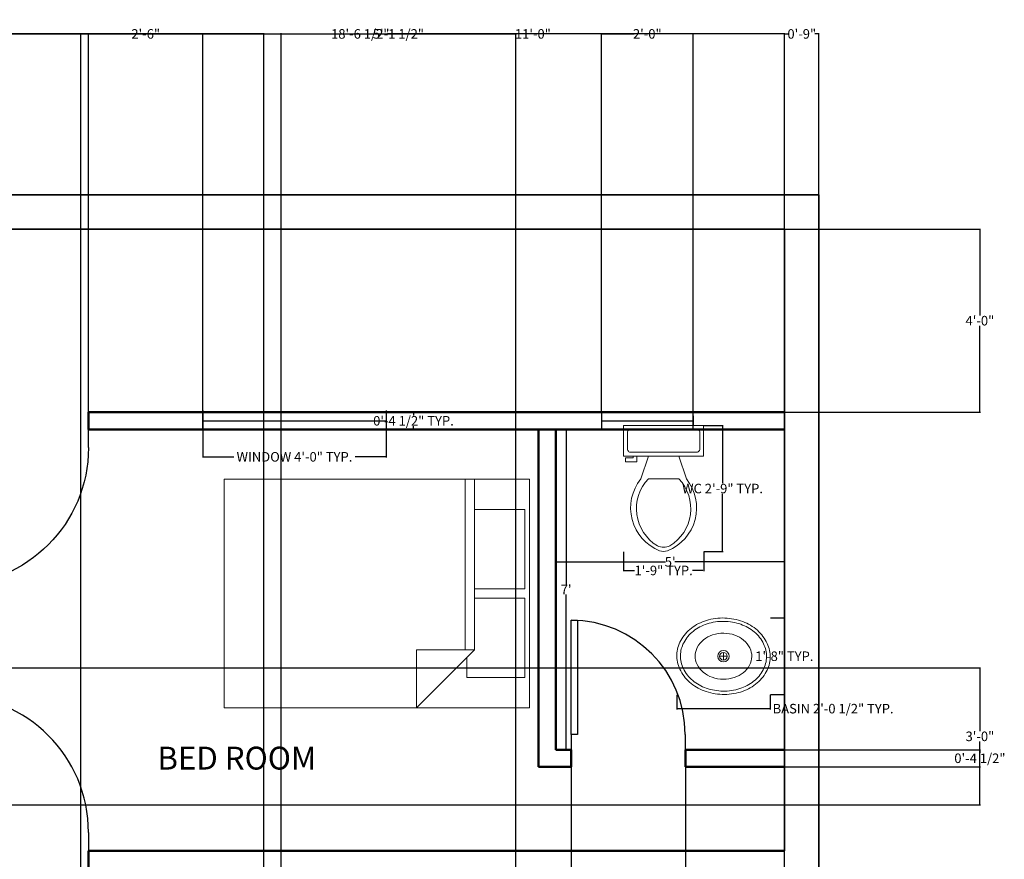
# Model space of a CAD drawing. Units: inches. Extents: x 594 to 1173, y 353 to 1285.
# Tile 6 of 6: x 914 to 1172, y 1065 to 1285. Entities that reach past the tile are written whole.
import ezdxf

# ---------------------------------------------------------------- set-up
doc = ezdxf.new("R2010")
doc.units = ezdxf.units.IN
doc.header["$MEASUREMENT"] = 0
for name, color, linetype, lineweight in [('A-ANNO-DIMS', 2, 'Continuous', 18), ('A-AREA-IDEN', 7, 'Continuous', 25), ('A-DOOR', 4, 'Continuous', 25), ('A-FLOR-FIXT', 9, 'Continuous', 18), ('A-FURN', 8, 'Continuous', 18), ('A-GLAZ', 4, 'Continuous', 25), ('A-WALL', 7, 'Continuous', 50), ('C-PROP', 7, 'Continuous', 35)]:
    doc.layers.add(name, color=color, linetype=linetype, lineweight=lineweight)
doc.styles.get("Standard").update_dxf_attribs({"font": 'arial.ttf'})
doc.dimstyles.get("Standard").update_dxf_attribs({"dimtxt": 2.5, "dimasz": 0.18, "dimexe": 0.18, "dimexo": 0.0625, "dimgap": 0.09, "dimtad": 0, "dimtih": 1, "dimtoh": 1, "dimzin": 0, "dimdsep": 46, "dimlunit": 3, "dimtxsty": 'Standard', "dimcen": 0.09, "dimadec": 0, "dimazin": 0, "dimtfac": 1, "dimtofl": 0, "dimtmove": 0, "dimatfit": 3, "dimfxl": 1, "dimtolj": 1, "dimtzin": 0, "dimarcsym": 0})

# ---------------------------------------------------------------- blocks, each defined once
blk = doc.blocks.new('*U4')
for p, q in [((0, 100), (0, 0)), ((900, 100), (900, 0)), ((0, 50), (900, 50))]:
    blk.add_line(p, q)
blk = doc.blocks.new('*U2')
for p, q in [((0, 0), (0, -100)), ((750, 0), (750, -100))]:
    blk.add_line(p, q)
blk.add_lwpolyline([(0, 0), (0, 750), (43.75, 750), (43.75, 0)], close=True)
blk.add_arc((0, 0), 750, 0, 90)
blk = doc.blocks.new('Bed - Queen')
for p, q in [((0, -80.00003), (0, 0)), ((0, 0), (59.99999, 0)), ((59.99999, 0), (59.99999, -80.00003)), ((7.99999, -1.2), (28.79998, -1.2)), ((7.99999, -14.4), (7.99999, -1.2)), ((28.79998, -1.2), (28.79998, -14.4)), ((31.19999, -1.2), (51.99999, -1.2)), ((31.19999, -14.4), (31.19999, -1.2)), ((51.99999, -1.2), (51.99999, -16.4)), ((0, -14.4), (44.8, -14.4)), ((59.99999, -29.6), (44.8, -14.4)), ((44.8, -14.4), (44.8, -29.6)), ((44.8, -16.8), (0, -16.8)), ((51.99999, -16.4), (46.79936, -16.4)), ((44.8, -29.6), (59.99999, -29.6)), ((59.99999, -80.00003), (0, -80.00003))]:
    blk.add_line(p, q)
blk = doc.blocks.new('Toilet - top')
for p, q in [((9.5, -6), (9.5, -2)), ((-10, -8.5), (-8, -8.5)), ((-10, -9.5), (-10, -8.5)), ((-7, -9.5), (-10, -9.5)), ((-8, -8.5), (-8, -8)), ((-7, -8), (-7, -9.5)), ((-4, -8), (-6, -14)), ((4, -8), (6, -14)), ((4, -14), (-4, -14))]:
    blk.add_line(p, q)
blk.add_lwpolyline([(10.5, -8), (10.5, 0), (-10.5, 0), (-10.5, -8)], close=True)
for points in [[(-9.5, -2), (-9.5, -6)], [(8.5, -1), (-8.5, -1)], [(-8.5, -7), (8.5, -7)]]:
    blk.add_lwpolyline(points)
for centre, radius, start, end in [((-8.62, -1.88), 0.884, 81.8699, 188.1301), ((8.62, -1.88), 0.884, 351.8699, 98.1301), ((-8.62, -6.12), 0.884, 171.8699, 278.1301), ((8.62, -6.12), 0.884, 261.8699, 8.1301), ((3.52, -21.58), 12.17, 141.4691, 247.9714), ((4.2, -21.82), 11.33, 136.3677, 238.9468), ((-3.52, -21.58), 12.17, 292.0284, 38.5307), ((-4.2, -21.82), 11.33, 301.053, 43.6321), ((0, -27.88), 4, 245.7318, 294.2682), ((0, -29), 4, 254.8605, 285.1395)]:
    blk.add_arc(centre, radius, start, end)
blk = doc.blocks.new('Sink - Oval top')
for p, q in [((-1, 0), (1, 0)), ((0, 1), (0, -1))]:
    blk.add_line(p, q)
for points in [[(-12.23, 0.39, 0.117634), (-11.46, -3.36, 0.104469), (-8.88, -6.8, 0.090016), (-5.08, -9.07, 0.08192), (-0.32, -10.02, 0.08192), (4.49, -9.38, 0.090016), (8.42, -7.36, 0.104469), (11.22, -4.09, 0.117634), (12.23, -0.39, 0.117634), (11.46, 3.36, 0.104469), (8.88, 6.8, 0.090016), (5.08, 9.07, 0.08192), (0.32, 10.02, 0.08192), (-4.49, 9.38, 0.090016), (-8.42, 7.36, 0.104469), (-11.22, 4.09, 0.117634)], [(-11.29, 0.16, 0.118622), (-10.52, -3.25, 0.104678), (-8.07, -6.36, 0.089562), (-4.54, -8.37, 0.081185), (-0.13, -9.15, 0.081185), (4.3, -8.49, 0.089562), (7.89, -6.58, 0.104678), (10.42, -3.55, 0.118622), (11.29, -0.16, 0.118622), (10.52, 3.25, 0.104678), (8.07, 6.36, 0.089562), (4.54, 8.37, 0.081185), (0.13, 9.15, 0.081185), (-4.3, 8.49, 0.089562), (-7.89, 6.58, 0.104678), (-10.42, 3.55, 0.118622)], [(-7.42, 0.08, 0.118283), (-6.91, -2.17, 0.104607), (-5.29, -4.21, 0.089718), (-2.97, -5.53, 0.081436), (-0.07, -6.04, 0.081436), (2.84, -5.59, 0.089718), (5.2, -4.33, 0.104607), (6.86, -2.32, 0.118283), (7.42, -0.08, 0.118283), (6.91, 2.17, 0.104607), (5.29, 4.21, 0.089718), (2.97, 5.53, 0.081436), (0.07, 6.04, 0.081436), (-2.84, 5.59, 0.089718), (-5.2, 4.33, 0.104607), (-6.86, 2.32, 0.118283)]]:
    blk.add_lwpolyline(points, format="xyb", close=True)
for radius in [1.5, 1]:
    blk.add_circle((0, 0), radius)
blk = doc.blocks.new('*D15')
at = {"layer": 'A-ANNO-DIMS', "color": 0, "lineweight": -2, "transparency": 16777216}
for p, q in [((1054.34, 1177.22), (1054.34, 1142.36)), ((1114.34, 1177.22), (1114.34, 1142.36)), ((1054.52, 1142.54), (1083.1, 1142.54)), ((1114.16, 1142.54), (1085.58, 1142.54))]:
    blk.add_line(p, q, dxfattribs=at)
at = {"layer": 'A-ANNO-DIMS', "color": 0, "transparency": 16777216}
for points in [[(1054.52, 1142.57), (1054.52, 1142.51), (1054.34, 1142.54)], [(1114.16, 1142.57), (1114.16, 1142.51), (1114.34, 1142.54)]]:
    blk.add_solid(points, dxfattribs=at)
at = {"layer": 'Defpoints', "color": 0, "transparency": 16777216}
for p in [(1054.34, 1177.28), (1114.34, 1177.28), (1054.34, 1142.54)]:
    blk.add_point(p, dxfattribs=at)
at = {"layer": 'A-ANNO-DIMS', "color": 0, "transparency": 16777216, "insert": (1084.34, 1142.54), "char_height": 2.5, "attachment_point": 5}
blk.add_mtext("\\A1;5'", dxfattribs=at)
blk = doc.blocks.new('*D16')
at = {"layer": 'A-ANNO-DIMS', "color": 0, "lineweight": -2, "transparency": 16777216}
for p, q in [((1054.4, 1177.28), (1057.24, 1177.28)), ((1057.06, 1177.1), (1057.06, 1136.62)), ((1057.06, 1093.46), (1057.06, 1133.94)), ((1054.4, 1093.28), (1057.24, 1093.28))]:
    blk.add_line(p, q, dxfattribs=at)
at = {"layer": 'A-ANNO-DIMS', "color": 0, "transparency": 16777216}
for points in [[(1057.03, 1177.1), (1057.09, 1177.1), (1057.06, 1177.28)], [(1057.03, 1093.46), (1057.09, 1093.46), (1057.06, 1093.28)]]:
    blk.add_solid(points, dxfattribs=at)
at = {"layer": 'Defpoints', "color": 0, "transparency": 16777216}
for p in [(1054.34, 1177.28), (1057.06, 1177.28), (1054.34, 1093.28)]:
    blk.add_point(p, dxfattribs=at)
at = {"layer": 'A-ANNO-DIMS', "color": 0, "transparency": 16777216, "insert": (1057.06, 1135.28), "char_height": 2.5, "attachment_point": 5}
blk.add_mtext("\\A1;7'", dxfattribs=at)
blk = doc.blocks.new('WIN-FRAME-48IN')
for p, q in [((0, 0), (0, 4.5)), ((0, 4.5), (48, 4.5)), ((48, 4.5), (48, 0))]:
    blk.add_line(p, q)
blk = doc.blocks.new('*D26')
at = {"layer": 'A-ANNO-DIMS', "color": 0, "lineweight": -2, "transparency": 16777216}
for p, q in [((1086.04, 1107.66), (1086.04, 1103.86)), ((1110.59, 1107.66), (1110.59, 1103.86)), ((1086.22, 1104.04), (1110.41, 1104.04)), ((1110.59, 1104.04), (1110.77, 1104.04))]:
    blk.add_line(p, q, dxfattribs=at)
at = {"layer": 'A-ANNO-DIMS', "color": 0, "transparency": 16777216}
for points in [[(1086.22, 1104.07), (1086.22, 1104.01), (1086.04, 1104.04)], [(1110.41, 1104.07), (1110.41, 1104.01), (1110.59, 1104.04)]]:
    blk.add_solid(points, dxfattribs=at)
at = {"layer": 'Defpoints', "color": 0, "transparency": 16777216}
for p in [(1086.04, 1107.72), (1110.59, 1107.72), (1110.59, 1104.04)]:
    blk.add_point(p, dxfattribs=at)
at = {"layer": 'A-ANNO-DIMS', "color": 0, "transparency": 16777216, "insert": (1127.06, 1104.04), "char_height": 2.5, "attachment_point": 5}
blk.add_mtext('\\A1;BASIN 2\'-0 1/2" TYP.', dxfattribs=at)
blk = doc.blocks.new('*D27')
at = {"layer": 'A-ANNO-DIMS', "color": 0, "lineweight": -2, "transparency": 16777216}
for p, q in [((1110.65, 1127.86), (1114.45, 1127.86)), ((1114.27, 1127.68), (1114.27, 1119.15)), ((1114.27, 1107.9), (1114.27, 1116.42)), ((1110.65, 1107.72), (1114.45, 1107.72))]:
    blk.add_line(p, q, dxfattribs=at)
at = {"layer": 'A-ANNO-DIMS', "color": 0, "transparency": 16777216}
for points in [[(1114.24, 1127.68), (1114.3, 1127.68), (1114.27, 1127.86)], [(1114.24, 1107.9), (1114.3, 1107.9), (1114.27, 1107.72)]]:
    blk.add_solid(points, dxfattribs=at)
at = {"layer": 'Defpoints', "color": 0, "transparency": 16777216}
for p in [(1110.59, 1127.86), (1114.27, 1127.86), (1110.59, 1107.72)]:
    blk.add_point(p, dxfattribs=at)
at = {"layer": 'A-ANNO-DIMS', "color": 0, "transparency": 16777216, "insert": (1114.27, 1117.79), "char_height": 2.5, "attachment_point": 5}
blk.add_mtext('\\A1;1\'-8" TYP.', dxfattribs=at)
blk = doc.blocks.new('*D28')
at = {"layer": 'A-ANNO-DIMS', "color": 0, "lineweight": -2, "transparency": 16777216}
for p, q in [((1093.18, 1178.28), (1098.25, 1178.28)), ((1098.07, 1178.1), (1098.07, 1163.14)), ((1098.07, 1145.42), (1098.07, 1160.38)), ((1093.18, 1145.24), (1098.25, 1145.24))]:
    blk.add_line(p, q, dxfattribs=at)
at = {"layer": 'A-ANNO-DIMS', "color": 0, "transparency": 16777216}
for points in [[(1098.04, 1178.1), (1098.1, 1178.1), (1098.07, 1178.28)], [(1098.04, 1145.42), (1098.1, 1145.42), (1098.07, 1145.24)]]:
    blk.add_solid(points, dxfattribs=at)
at = {"layer": 'Defpoints', "color": 0, "transparency": 16777216}
for p in [(1093.12, 1178.28), (1098.07, 1178.28), (1093.12, 1145.24)]:
    blk.add_point(p, dxfattribs=at)
at = {"layer": 'A-ANNO-DIMS', "color": 0, "transparency": 16777216, "insert": (1098.07, 1161.76), "char_height": 2.5, "attachment_point": 5}
blk.add_mtext('\\A1;WC 2\'-9" TYP.', dxfattribs=at)
blk = doc.blocks.new('*D29')
at = {"layer": 'A-ANNO-DIMS', "color": 0, "lineweight": -2, "transparency": 16777216}
for p, q in [((1072.12, 1145.17), (1072.12, 1140.1)), ((1093.12, 1145.17), (1093.12, 1140.1)), ((1072.3, 1140.28), (1075.02, 1140.28)), ((1092.94, 1140.28), (1090.21, 1140.28))]:
    blk.add_line(p, q, dxfattribs=at)
at = {"layer": 'A-ANNO-DIMS', "color": 0, "transparency": 16777216}
for points in [[(1072.3, 1140.31), (1072.3, 1140.25), (1072.12, 1140.28)], [(1092.94, 1140.31), (1092.94, 1140.25), (1093.12, 1140.28)]]:
    blk.add_solid(points, dxfattribs=at)
at = {"layer": 'Defpoints', "color": 0, "transparency": 16777216}
for p in [(1072.12, 1145.24), (1093.12, 1145.24), (1093.12, 1140.28)]:
    blk.add_point(p, dxfattribs=at)
at = {"layer": 'A-ANNO-DIMS', "color": 0, "transparency": 16777216, "insert": (1082.62, 1140.28), "char_height": 2.5, "attachment_point": 5}
blk.add_mtext('\\A1;1\'-9" TYP.', dxfattribs=at)
blk = doc.blocks.new('*D30')
at = {"layer": 'A-ANNO-DIMS', "color": 0, "lineweight": -2, "transparency": 16777216}
for p, q in [((961.84, 1177.22), (961.84, 1169.9)), ((1009.84, 1177.22), (1009.84, 1169.9)), ((962.02, 1170.08), (969.93, 1170.08)), ((1009.66, 1170.08), (1001.74, 1170.08))]:
    blk.add_line(p, q, dxfattribs=at)
at = {"layer": 'A-ANNO-DIMS', "color": 0, "transparency": 16777216}
for points in [[(962.02, 1170.11), (962.02, 1170.05), (961.84, 1170.08)], [(1009.66, 1170.11), (1009.66, 1170.05), (1009.84, 1170.08)]]:
    blk.add_solid(points, dxfattribs=at)
at = {"layer": 'Defpoints', "color": 0, "transparency": 16777216}
for p in [(961.84, 1177.28), (1009.84, 1177.28), (1009.84, 1170.08)]:
    blk.add_point(p, dxfattribs=at)
at = {"layer": 'A-ANNO-DIMS', "color": 0, "transparency": 16777216, "insert": (985.84, 1170.08), "char_height": 2.5, "attachment_point": 5}
blk.add_mtext('\\A1;WINDOW 4\'-0" TYP.', dxfattribs=at)
blk = doc.blocks.new('*D31')
at = {"layer": 'A-ANNO-DIMS', "color": 0, "lineweight": -2, "transparency": 16777216}
for p, q in [((1009.9, 1181.78), (1017.22, 1181.78)), ((1017.04, 1181.6), (1017.04, 1180.92)), ((1009.9, 1177.28), (1017.22, 1177.28)), ((1017.04, 1177.46), (1017.04, 1178.15))]:
    blk.add_line(p, q, dxfattribs=at)
at = {"layer": 'A-ANNO-DIMS', "color": 0, "transparency": 16777216}
for points in [[(1017.01, 1181.6), (1017.07, 1181.6), (1017.04, 1181.78)], [(1017.01, 1177.46), (1017.07, 1177.46), (1017.04, 1177.28)]]:
    blk.add_solid(points, dxfattribs=at)
at = {"layer": 'Defpoints', "color": 0, "transparency": 16777216}
for p in [(1009.84, 1181.78), (1017.04, 1181.78), (1009.84, 1177.28)]:
    blk.add_point(p, dxfattribs=at)
at = {"layer": 'A-ANNO-DIMS', "color": 0, "transparency": 16777216, "insert": (1017.04, 1179.53), "char_height": 2.5, "attachment_point": 5}
blk.add_mtext('\\A1;0\'-4 1/2" TYP.', dxfattribs=at)
blk = doc.blocks.new('*D50')
at = {"layer": 'A-ANNO-DIMS', "color": 0, "lineweight": -2, "transparency": 16777216}
for p, q in [((891.84, 1177.35), (891.84, 1281.16)), ((892.02, 1280.98), (995.91, 1280.98)), ((1114.16, 1280.98), (1010.27, 1280.98)), ((1114.34, 1177.35), (1114.34, 1281.16))]:
    blk.add_line(p, q, dxfattribs=at)
at = {"layer": 'A-ANNO-DIMS', "color": 0, "transparency": 16777216}
for points in [[(892.02, 1281.01), (892.02, 1280.95), (891.84, 1280.98)], [(1114.16, 1281.01), (1114.16, 1280.95), (1114.34, 1280.98)]]:
    blk.add_solid(points, dxfattribs=at)
at = {"layer": 'Defpoints', "color": 0, "transparency": 16777216}
for p in [(1114.34, 1280.98), (891.84, 1177.28), (1114.34, 1177.28)]:
    blk.add_point(p, dxfattribs=at)
at = {"layer": 'A-ANNO-DIMS', "color": 0, "transparency": 16777216, "insert": (1003.09, 1280.98), "char_height": 2.5, "attachment_point": 5}
blk.add_mtext('\\A1;18\'-6 1/2"', dxfattribs=at)
blk = doc.blocks.new('*D52')
at = {"layer": 'A-ANNO-DIMS', "color": 0, "lineweight": -2, "transparency": 16777216}
for p, q in [((982.34, 968.85), (982.34, 1281.16)), ((982.52, 1280.98), (1044.07, 1280.98)), ((1114.16, 1280.98), (1052.6, 1280.98)), ((1114.34, 848.85), (1114.34, 1281.16))]:
    blk.add_line(p, q, dxfattribs=at)
at = {"layer": 'A-ANNO-DIMS', "color": 0, "transparency": 16777216}
for points in [[(982.52, 1281.01), (982.52, 1280.95), (982.34, 1280.98)], [(1114.16, 1281.01), (1114.16, 1280.95), (1114.34, 1280.98)]]:
    blk.add_solid(points, dxfattribs=at)
at = {"layer": 'Defpoints', "color": 0, "transparency": 16777216}
for p in [(1114.34, 1280.98), (982.34, 968.78), (1114.34, 848.78)]:
    blk.add_point(p, dxfattribs=at)
at = {"layer": 'A-ANNO-DIMS', "color": 0, "transparency": 16777216, "insert": (1048.34, 1280.98), "char_height": 2.5, "attachment_point": 5}
blk.add_mtext('\\A1;11\'-0"', dxfattribs=at)
blk = doc.blocks.new('*D54')
at = {"layer": 'A-ANNO-DIMS', "color": 0, "lineweight": -2, "transparency": 16777216}
for p, q in [((982.34, 1062.35), (982.34, 1281.16)), ((982.52, 1280.98), (1006.76, 1280.98)), ((1043.66, 1280.98), (1019.41, 1280.98)), ((1043.84, 1062.35), (1043.84, 1281.16))]:
    blk.add_line(p, q, dxfattribs=at)
at = {"layer": 'A-ANNO-DIMS', "color": 0, "transparency": 16777216}
for points in [[(982.52, 1281.01), (982.52, 1280.95), (982.34, 1280.98)], [(1043.66, 1281.01), (1043.66, 1280.95), (1043.84, 1280.98)]]:
    blk.add_solid(points, dxfattribs=at)
at = {"layer": 'Defpoints', "color": 0, "transparency": 16777216}
for p in [(1043.84, 1280.98), (982.34, 1062.28), (1043.84, 1062.28)]:
    blk.add_point(p, dxfattribs=at)
at = {"layer": 'A-ANNO-DIMS', "color": 0, "transparency": 16777216, "insert": (1013.09, 1280.98), "char_height": 2.5, "attachment_point": 5}
blk.add_mtext('\\A1;5\'-1 1/2"', dxfattribs=at)
blk = doc.blocks.new('*D57')
at = {"layer": 'A-ANNO-DIMS', "color": 0, "lineweight": -2, "transparency": 16777216}
for p, q in [((1114.4, 1229.78), (1165.72, 1229.78)), ((1165.54, 1229.6), (1165.54, 1207.15)), ((1165.54, 1181.96), (1165.54, 1204.42)), ((1114.4, 1181.78), (1165.72, 1181.78))]:
    blk.add_line(p, q, dxfattribs=at)
at = {"layer": 'A-ANNO-DIMS', "color": 0, "transparency": 16777216}
for points in [[(1165.51, 1229.6), (1165.57, 1229.6), (1165.54, 1229.78)], [(1165.51, 1181.96), (1165.57, 1181.96), (1165.54, 1181.78)]]:
    blk.add_solid(points, dxfattribs=at)
at = {"layer": 'Defpoints', "color": 0, "transparency": 16777216}
for p in [(1114.34, 1229.78), (1165.54, 1229.78), (1114.34, 1181.78)]:
    blk.add_point(p, dxfattribs=at)
at = {"layer": 'A-ANNO-DIMS', "color": 0, "transparency": 16777216, "insert": (1165.54, 1205.78), "char_height": 2.5, "attachment_point": 5}
blk.add_mtext('\\A1;4\'-0"', dxfattribs=at)
blk = doc.blocks.new('*D58')
at = {"layer": 'A-ANNO-DIMS', "color": 0, "lineweight": -2, "transparency": 16777216}
for p, q in [((829.34, 647.85), (829.34, 1281.16)), ((829.52, 1280.98), (873.26, 1280.98)), ((929.66, 1280.98), (885.91, 1280.98)), ((929.84, 647.85), (929.84, 1281.16))]:
    blk.add_line(p, q, dxfattribs=at)
at = {"layer": 'A-ANNO-DIMS', "color": 0, "transparency": 16777216}
for points in [[(829.52, 1281.01), (829.52, 1280.95), (829.34, 1280.98)], [(929.66, 1281.01), (929.66, 1280.95), (929.84, 1280.98)]]:
    blk.add_solid(points, dxfattribs=at)
at = {"layer": 'Defpoints', "color": 0, "transparency": 16777216}
for p in [(929.84, 1280.98), (829.34, 647.78), (929.84, 647.78)]:
    blk.add_point(p, dxfattribs=at)
at = {"layer": 'A-ANNO-DIMS', "color": 0, "transparency": 16777216, "insert": (879.59, 1280.98), "char_height": 2.5, "attachment_point": 5}
blk.add_mtext('\\A1;8\'-4 1/2"', dxfattribs=at)
blk = doc.blocks.new('*D61')
at = {"layer": 'A-ANNO-DIMS', "color": 0, "lineweight": -2, "transparency": 16777216}
for p, q in [((728.84, 1062.35), (728.84, 1281.16)), ((729.02, 1280.98), (848.93, 1280.98)), ((977.66, 1280.98), (857.74, 1280.98)), ((977.84, 1062.35), (977.84, 1281.16))]:
    blk.add_line(p, q, dxfattribs=at)
at = {"layer": 'A-ANNO-DIMS', "color": 0, "transparency": 16777216}
for points in [[(729.02, 1281.01), (729.02, 1280.95), (728.84, 1280.98)], [(977.66, 1281.01), (977.66, 1280.95), (977.84, 1280.98)]]:
    blk.add_solid(points, dxfattribs=at)
at = {"layer": 'Defpoints', "color": 0, "transparency": 16777216}
for p in [(977.84, 1280.98), (728.84, 1062.28), (977.84, 1062.28)]:
    blk.add_point(p, dxfattribs=at)
at = {"layer": 'A-ANNO-DIMS', "color": 0, "transparency": 16777216, "insert": (853.34, 1280.98), "char_height": 2.5, "attachment_point": 5}
blk.add_mtext('\\A1;20\'-9"', dxfattribs=at)
blk = doc.blocks.new('*D65')
at = {"layer": 'A-ANNO-DIMS', "color": 0, "lineweight": -2, "transparency": 16777216}
for p, q in [((1114.34, 1229.85), (1114.34, 1281.16)), ((1114.52, 1280.98), (1115.42, 1280.98)), ((1123.16, 1280.98), (1122.25, 1280.98)), ((1123.34, 1238.85), (1123.34, 1281.16))]:
    blk.add_line(p, q, dxfattribs=at)
at = {"layer": 'A-ANNO-DIMS', "color": 0, "transparency": 16777216}
for points in [[(1114.52, 1281.01), (1114.52, 1280.95), (1114.34, 1280.98)], [(1123.16, 1281.01), (1123.16, 1280.95), (1123.34, 1280.98)]]:
    blk.add_solid(points, dxfattribs=at)
at = {"layer": 'Defpoints', "color": 0, "transparency": 16777216}
for p in [(1123.34, 1280.98), (1123.34, 1238.78), (1114.34, 1229.78)]:
    blk.add_point(p, dxfattribs=at)
at = {"layer": 'A-ANNO-DIMS', "color": 0, "transparency": 16777216, "insert": (1118.84, 1280.98), "char_height": 2.5, "attachment_point": 5}
blk.add_mtext('\\A1;0\'-9"', dxfattribs=at)
blk = doc.blocks.new('*D66')
at = {"layer": 'A-ANNO-DIMS', "color": 0, "lineweight": -2, "transparency": 16777216}
for p, q in [((1114.4, 1093.28), (1165.72, 1093.28)), ((1165.54, 1093.1), (1165.54, 1092.42)), ((1165.54, 1088.96), (1165.54, 1089.65)), ((1114.4, 1088.78), (1165.72, 1088.78))]:
    blk.add_line(p, q, dxfattribs=at)
at = {"layer": 'A-ANNO-DIMS', "color": 0, "transparency": 16777216}
for points in [[(1165.51, 1093.1), (1165.57, 1093.1), (1165.54, 1093.28)], [(1165.51, 1088.96), (1165.57, 1088.96), (1165.54, 1088.78)]]:
    blk.add_solid(points, dxfattribs=at)
at = {"layer": 'Defpoints', "color": 0, "transparency": 16777216}
for p in [(1114.34, 1093.28), (1165.54, 1093.28), (1114.34, 1088.78)]:
    blk.add_point(p, dxfattribs=at)
at = {"layer": 'A-ANNO-DIMS', "color": 0, "transparency": 16777216, "insert": (1165.54, 1091.03), "char_height": 2.5, "attachment_point": 5}
blk.add_mtext('\\A1;0\'-4 1/2"', dxfattribs=at)
blk = doc.blocks.new('*D67')
at = {"layer": 'A-ANNO-DIMS', "color": 0, "lineweight": -2, "transparency": 16777216}
for p, q in [((1058.34, 1093.22), (1058.34, 356.4)), ((1088.34, 1093.22), (1088.34, 356.4)), ((1058.52, 356.58), (1069.9, 356.58)), ((1088.16, 356.58), (1076.77, 356.58))]:
    blk.add_line(p, q, dxfattribs=at)
at = {"layer": 'A-ANNO-DIMS', "color": 0, "transparency": 16777216}
for points in [[(1058.52, 356.61), (1058.52, 356.55), (1058.34, 356.58)], [(1088.16, 356.61), (1088.16, 356.55), (1088.34, 356.58)]]:
    blk.add_solid(points, dxfattribs=at)
at = {"layer": 'Defpoints', "color": 0, "transparency": 16777216}
for p in [(1058.34, 1093.28), (1088.34, 1093.28), (1058.34, 356.58)]:
    blk.add_point(p, dxfattribs=at)
at = {"layer": 'A-ANNO-DIMS', "color": 0, "transparency": 16777216, "insert": (1073.34, 356.58), "char_height": 2.5, "attachment_point": 5}
blk.add_mtext('\\A1;2\'-6"', dxfattribs=at)
blk = doc.blocks.new('*D77')
at = {"layer": 'A-ANNO-DIMS', "color": 0, "lineweight": -2, "transparency": 16777216}
for p, q in [((931.84, 1181.85), (931.84, 1281.16)), ((932.02, 1280.98), (943.4, 1280.98)), ((961.66, 1280.98), (950.27, 1280.98)), ((961.84, 1181.85), (961.84, 1281.16))]:
    blk.add_line(p, q, dxfattribs=at)
at = {"layer": 'A-ANNO-DIMS', "color": 0, "transparency": 16777216}
for points in [[(932.02, 1281.01), (932.02, 1280.95), (931.84, 1280.98)], [(961.66, 1281.01), (961.66, 1280.95), (961.84, 1280.98)]]:
    blk.add_solid(points, dxfattribs=at)
at = {"layer": 'Defpoints', "color": 0, "transparency": 16777216}
for p in [(961.84, 1280.98), (931.84, 1181.78), (961.84, 1181.78)]:
    blk.add_point(p, dxfattribs=at)
at = {"layer": 'A-ANNO-DIMS', "color": 0, "transparency": 16777216, "insert": (946.84, 1280.98), "char_height": 2.5, "attachment_point": 5}
blk.add_mtext('\\A1;2\'-6"', dxfattribs=at)
blk = doc.blocks.new('*D78')
at = {"layer": 'A-ANNO-DIMS', "color": 0, "lineweight": -2, "transparency": 16777216}
for p, q in [((1066.34, 1181.85), (1066.34, 1281.16)), ((1066.52, 1280.98), (1074.9, 1280.98)), ((1090.16, 1280.98), (1081.77, 1280.98)), ((1090.34, 1181.85), (1090.34, 1281.16))]:
    blk.add_line(p, q, dxfattribs=at)
at = {"layer": 'A-ANNO-DIMS', "color": 0, "transparency": 16777216}
for points in [[(1066.52, 1281.01), (1066.52, 1280.95), (1066.34, 1280.98)], [(1090.16, 1281.01), (1090.16, 1280.95), (1090.34, 1280.98)]]:
    blk.add_solid(points, dxfattribs=at)
at = {"layer": 'Defpoints', "color": 0, "transparency": 16777216}
for p in [(1090.34, 1280.98), (1066.34, 1181.78), (1090.34, 1181.78)]:
    blk.add_point(p, dxfattribs=at)
at = {"layer": 'A-ANNO-DIMS', "color": 0, "transparency": 16777216, "insert": (1078.34, 1280.98), "char_height": 2.5, "attachment_point": 5}
blk.add_mtext('\\A1;2\'-0"', dxfattribs=at)
blk = doc.blocks.new('*D82')
at = {"layer": 'A-ANNO-DIMS', "color": 0, "lineweight": -2, "transparency": 16777216}
for p, q in [((724.4, 1114.78), (1165.72, 1114.78)), ((1165.54, 1114.6), (1165.54, 1098.15)), ((1165.54, 1078.96), (1165.54, 1095.42)), ((724.4, 1078.78), (1165.72, 1078.78))]:
    blk.add_line(p, q, dxfattribs=at)
at = {"layer": 'A-ANNO-DIMS', "color": 0, "transparency": 16777216}
for points in [[(1165.51, 1114.6), (1165.57, 1114.6), (1165.54, 1114.78)], [(1165.51, 1078.96), (1165.57, 1078.96), (1165.54, 1078.78)]]:
    blk.add_solid(points, dxfattribs=at)
at = {"layer": 'Defpoints', "color": 0, "transparency": 16777216}
for p in [(724.34, 1114.78), (1165.54, 1114.78), (724.34, 1078.78)]:
    blk.add_point(p, dxfattribs=at)
at = {"layer": 'A-ANNO-DIMS', "color": 0, "transparency": 16777216, "insert": (1165.54, 1096.78), "char_height": 2.5, "attachment_point": 5}
blk.add_mtext('\\A1;3\'-0"', dxfattribs=at)

msp = doc.modelspace()

# ---------------------------------------------------------------- linework, layer by layer
at = {"layer": 'A-GLAZ'}
for p, q in [((1090.337, 1181.783), (1066.337, 1181.783)), ((1066.337, 1181.783), (1066.337, 1177.283)), ((1090.337, 1177.283), (1090.337, 1181.783))]:
    msp.add_line(p, q, dxfattribs=at)
at = {"layer": 'A-WALL'}
for p, q in [((1114.337, 1181.783), (931.837, 1181.783)), ((931.837, 1181.783), (931.837, 1177.283)), ((1114.337, 1177.283), (931.837, 1177.283)), ((1049.837, 1088.783), (1049.837, 1177.283)), ((1054.337, 1093.283), (1054.337, 1177.283)), ((1058.337, 1093.283), (1054.337, 1093.283)), ((1058.337, 1093.283), (1058.337, 1088.783)), ((1114.337, 1093.283), (1088.27, 1093.283)), ((1088.337, 1088.783), (1088.337, 1093.283)), ((1058.337, 1088.783), (1049.837, 1088.783)), ((1114.337, 1088.783), (1088.337, 1088.783)), ((931.837, 1062.283), (931.837, 1066.783)), ((931.837, 1066.783), (1114.337, 1066.783)), ((1054.337, 1066.783), (1114.337, 1066.783))]:
    msp.add_line(p, q, dxfattribs=at)
at = {"layer": 'C-PROP'}
for p, q in [((1123.337, 1238.783), (643.337, 1238.783)), ((1123.337, 398.783), (1123.337, 1238.783)), ((1114.337, 1229.783), (652.337, 1229.783)), ((1114.337, 1066.783), (1114.337, 1229.783))]:
    msp.add_line(p, q, dxfattribs=at)

# ---------------------------------------------------------------- block references
at = {"layer": 'A-DOOR', "xscale": -0.0479999999999999, "yscale": 0.0479999999999999, "zscale": 0.0479999999999999, "rotation": 180}
msp.add_blockref('*U2', (895.837, 1172.483), dxfattribs=at)
at = {"layer": 'A-DOOR'}
for p, xscale, yscale, zscale in [((1058.337, 1097.274), 0.0399114063142643, 0.0399114063142643, 0.0399114063142643), ((895.837, 1071.583), 0.0479999999999999, 0.0479999999999999, 0.0479999999999999)]:
    msp.add_blockref('*U2', p, dxfattribs=dict(at, xscale=xscale, yscale=yscale, zscale=zscale))
at = {"layer": 'A-FLOR-FIXT'}
for name, p in [('Toilet - top', (1082.616, 1178.283)), ('Sink - Oval top', (1098.312, 1117.787))]:
    msp.add_blockref(name, p, dxfattribs=at)
at = {"layer": 'A-FURN', "rotation": 270}
msp.add_blockref('Bed - Queen', (1047.431, 1164.233), dxfattribs=at)
at = {"layer": 'A-GLAZ'}
for p, xscale, yscale, zscale in [((961.837, 1176.866), 0.0533333333333332, 0.0533333333333332, 0.0533333333333332), ((1066.337, 1178.199), 0.0266666666666666, 0.0266666666666666, 0.0266666666666666)]:
    msp.add_blockref('*U4', p, dxfattribs=dict(at, xscale=xscale, yscale=yscale, zscale=zscale))
msp.add_blockref('WIN-FRAME-48IN', (961.837, 1177.283), dxfattribs=at)

# ---------------------------------------------------------------- texts
at = {"layer": 'A-AREA-IDEN'}
msp.add_text('BED ROOM', height=6, dxfattribs=at).set_placement((949.908, 1088.067))

# ---------------------------------------------------------------- dimensions: what is measured, and where the dimension line sits
at = {"layer": 'A-ANNO-DIMS'}
for base, p1, p2, override, picture, middle in [((929.837, 1280.983), (829.337, 647.783), (929.837, 647.783), {"dimdec": 1, "dimlfac": 1, "dimrnd": 0, "dimzin": 1, "dimdsep": 46, "dimlunit": 4, "dimfrac": 2}, '*D58', (879.587, 1280.983)), ((1114.337, 1280.983), (891.837, 1177.283), (1114.337, 1177.283), {"dimdec": 1, "dimlfac": 1, "dimrnd": 0, "dimzin": 1, "dimdsep": 46, "dimlunit": 4, "dimfrac": 2}, '*D50', (1003.087, 1280.983)), ((1043.837, 1280.983), (982.337, 1062.283), (1043.837, 1062.283), {"dimdec": 1, "dimlfac": 1, "dimrnd": 0, "dimzin": 1, "dimdsep": 46, "dimlunit": 4, "dimfrac": 2}, '*D54', (1013.087, 1280.983)), ((977.837, 1280.983), (728.837, 1062.283), (977.837, 1062.283), {"dimdec": 1, "dimlfac": 1, "dimrnd": 0, "dimzin": 1, "dimdsep": 46, "dimlunit": 4, "dimfrac": 2}, '*D61', (853.337, 1280.983)), ((961.837, 1280.983), (931.837, 1181.783), (961.837, 1181.783), {"dimdec": 1, "dimlfac": 1, "dimrnd": 0, "dimzin": 1, "dimdsep": 46, "dimlunit": 4, "dimfrac": 2}, '*D77', (946.837, 1280.983)), ((1114.337, 1280.983), (982.337, 968.783), (1114.337, 848.783), {"dimdec": 1, "dimlfac": 1, "dimrnd": 0, "dimzin": 1, "dimdsep": 46, "dimlunit": 4, "dimfrac": 2}, '*D52', (1048.337, 1280.983)), ((1090.337, 1280.983), (1066.337, 1181.783), (1090.337, 1181.783), {"dimdec": 1, "dimlfac": 1, "dimrnd": 0, "dimzin": 1, "dimdsep": 46, "dimlunit": 4, "dimfrac": 2}, '*D78', (1078.337, 1280.983)), ((1123.337, 1280.983), (1114.337, 1229.783), (1123.337, 1238.783), {"dimdec": 1, "dimlfac": 1, "dimrnd": 0, "dimzin": 1, "dimdsep": 46, "dimlunit": 4, "dimfrac": 2}, '*D65', (1118.837, 1280.983)), ((1054.337, 1142.541), (1114.337, 1177.283), (1054.337, 1177.283), {"dimclrd": 0, "dimclre": 0, "dimclrt": 0}, '*D15', (1084.337, 1142.541)), ((1058.337, 356.583), (1088.337, 1093.283), (1058.337, 1093.283), {"dimdec": 1, "dimlfac": 1, "dimrnd": 0, "dimzin": 1, "dimdsep": 46, "dimlunit": 4, "dimfrac": 2}, '*D67', (1073.337, 356.583))]:
    dim = msp.add_linear_dim(base=base, p1=p1, p2=p2, dimstyle='Standard', override=override, dxfattribs=at)
    dim.commit()
    dim.dimension.update_dxf_attribs({"geometry": picture, "text_midpoint": middle})
for base, p1, p2, override, picture, middle in [((1165.537, 1229.783), (1114.337, 1181.783), (1114.337, 1229.783), {"dimdec": 1, "dimlfac": 1, "dimrnd": 0, "dimzin": 1, "dimdsep": 46, "dimlunit": 4, "dimfrac": 2}, '*D57', (1165.537, 1205.783)), ((1057.057, 1177.283), (1054.337, 1093.283), (1054.337, 1177.283), {"dimclrd": 0, "dimclre": 0, "dimclrt": 0}, '*D16', (1057.057, 1135.283)), ((1165.537, 1114.783), (724.337, 1078.783), (724.337, 1114.783), {"dimdec": 1, "dimlfac": 1, "dimrnd": 0, "dimzin": 1, "dimdsep": 46, "dimlunit": 4, "dimfrac": 2}, '*D82', (1165.537, 1096.783)), ((1165.537, 1093.283), (1114.337, 1088.783), (1114.337, 1093.283), {"dimdec": 1, "dimlfac": 1, "dimrnd": 0, "dimzin": 1, "dimdsep": 46, "dimlunit": 4, "dimfrac": 2}, '*D66', (1165.537, 1091.033))]:
    dim = msp.add_linear_dim(base=base, p1=p1, p2=p2, angle=90, dimstyle='Standard', override=override, dxfattribs=at)
    dim.commit()
    dim.dimension.update_dxf_attribs({"geometry": picture, "text_midpoint": middle})
for base, p1, p2, text, picture, middle in [((1017.037, 1181.783), (1009.837, 1177.283), (1009.837, 1181.783), '<> TYP.', '*D31', (1017.037, 1179.533)), ((1098.073, 1178.283), (1093.116, 1145.236), (1093.116, 1178.283), 'WC <> TYP.', '*D28', (1098.073, 1161.759)), ((1114.27, 1127.856), (1110.587, 1107.719), (1110.587, 1127.856), '<> TYP.', '*D27', (1114.27, 1117.787))]:
    dim = msp.add_linear_dim(base=base, p1=p1, p2=p2, angle=90, text=text, dimstyle='Standard', override={"dimdec": 1, "dimlfac": 1, "dimrnd": 0, "dimzin": 1, "dimdsep": 46, "dimlunit": 4, "dimfrac": 2}, dxfattribs=at)
    dim.commit()
    dim.dimension.update_dxf_attribs({"geometry": picture, "text_midpoint": middle})
for base, p1, p2, text, picture, middle in [((1009.837, 1170.083), (961.837, 1177.283), (1009.837, 1177.283), 'WINDOW <> TYP.', '*D30', (985.837, 1170.083)), ((1093.116, 1140.279), (1072.116, 1145.236), (1093.116, 1145.236), '<> TYP.', '*D29', (1082.616, 1140.279)), ((1110.5874, 1104.0365), (1086.0365, 1107.7191), (1110.5874, 1107.7191), 'BASIN <> TYP.', '*D26', (1127.0596, 1104.0365))]:
    dim = msp.add_linear_dim(base=base, p1=p1, p2=p2, text=text, dimstyle='Standard', override={"dimdec": 1, "dimlfac": 1, "dimrnd": 0, "dimzin": 1, "dimdsep": 46, "dimlunit": 4, "dimfrac": 2}, dxfattribs=at)
    dim.commit()
    dim.dimension.update_dxf_attribs({"geometry": picture, "text_midpoint": middle})

doc.saveas('drawing.dxf')
